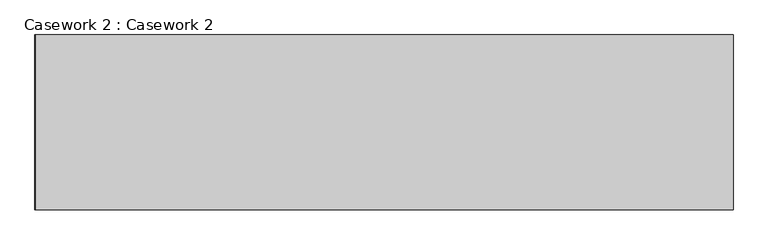
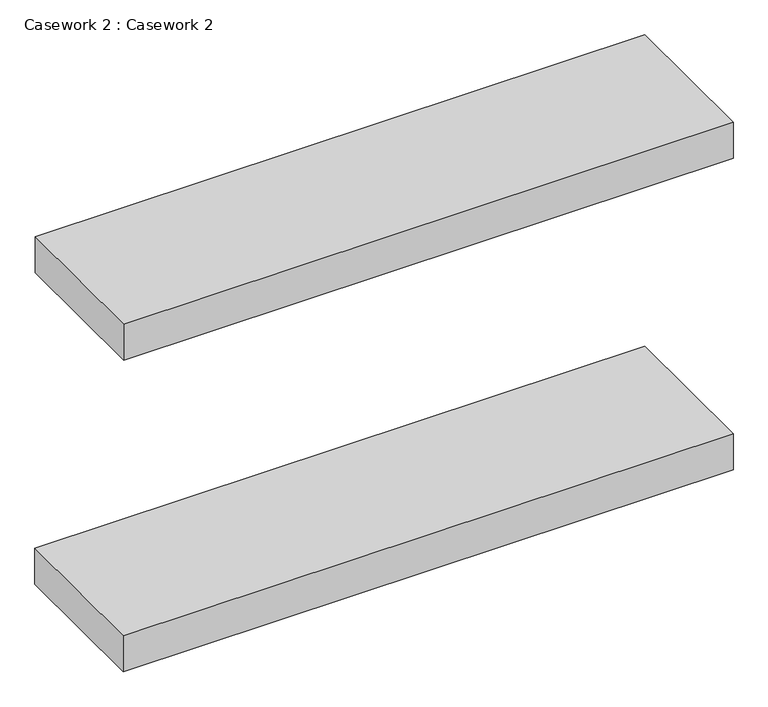
"""IFC4 building model written with IfcOpenShell, lengths in millimetres: furniture geometry, Casework 2 : Casework 2."""

from ifc_helpers import new_model, si_unit, frame, origin, place, context, project, spatial, polyline, outline, extrude, source, transform, mapped, element, save


def casework_2_casework_2_475e0740(model_context):
    return source(origin(), model_context, "Body", "SweptSolid", [
        extrude(outline(polyline([(-16087.5794706, -1453.6741596), (-21370.6794706, -1453.6741596), (-21370.6794706, -132.2741596), (-16087.5794706, -132.2741596), (-16087.5794706, -1453.6741596)])), frame((0.0, 0.0, 2820.0), z_axis=(0.0, 0.0, 1.0), x_axis=(1.0, 0.0, 0.0)), (0.0, 0.0, 1.0), 330.0),
        extrude(outline(polyline([(-16087.5794706, -1453.6741596), (-21365.6794706, -1453.6741596), (-21365.6794706, -132.2741596), (-16087.5794706, -132.2741596), (-16087.5794706, -1453.6741596)])), frame((0.0, 0.0, 5670.0), z_axis=(0.0, 0.0, 1.0), x_axis=(1.0, 0.0, 0.0)), (0.0, 0.0, 1.0), 330.0),
    ])


if __name__ == "__main__":
    model = new_model("IFC4")
    model_context = context("Model", 3, world=origin())
    ifc_project = project(units=[si_unit("LENGTHUNIT", "METRE", prefix="MILLI")], contexts=[model_context])
    site = spatial("IfcSite", under=ifc_project)
    building = spatial("IfcBuilding", under=site)
    placement = place(None, origin())
    casework_2_casework_2_shape = casework_2_casework_2_475e0740(model_context)
    element("IfcFurniture", 1, ObjectType="Casework 2 : Casework 2", at=placement, inside=building, context=model_context, shape_type="MappedRepresentation", body=[
        mapped(casework_2_casework_2_shape, transform((0.0, 0.0, 0.0), x_axis=(1.0, 0.0, 0.0), y_axis=(0.0, 1.0, 0.0), z_axis=(0.0, 0.0, 1.0))),
    ])
    save(model, "model.ifc")
